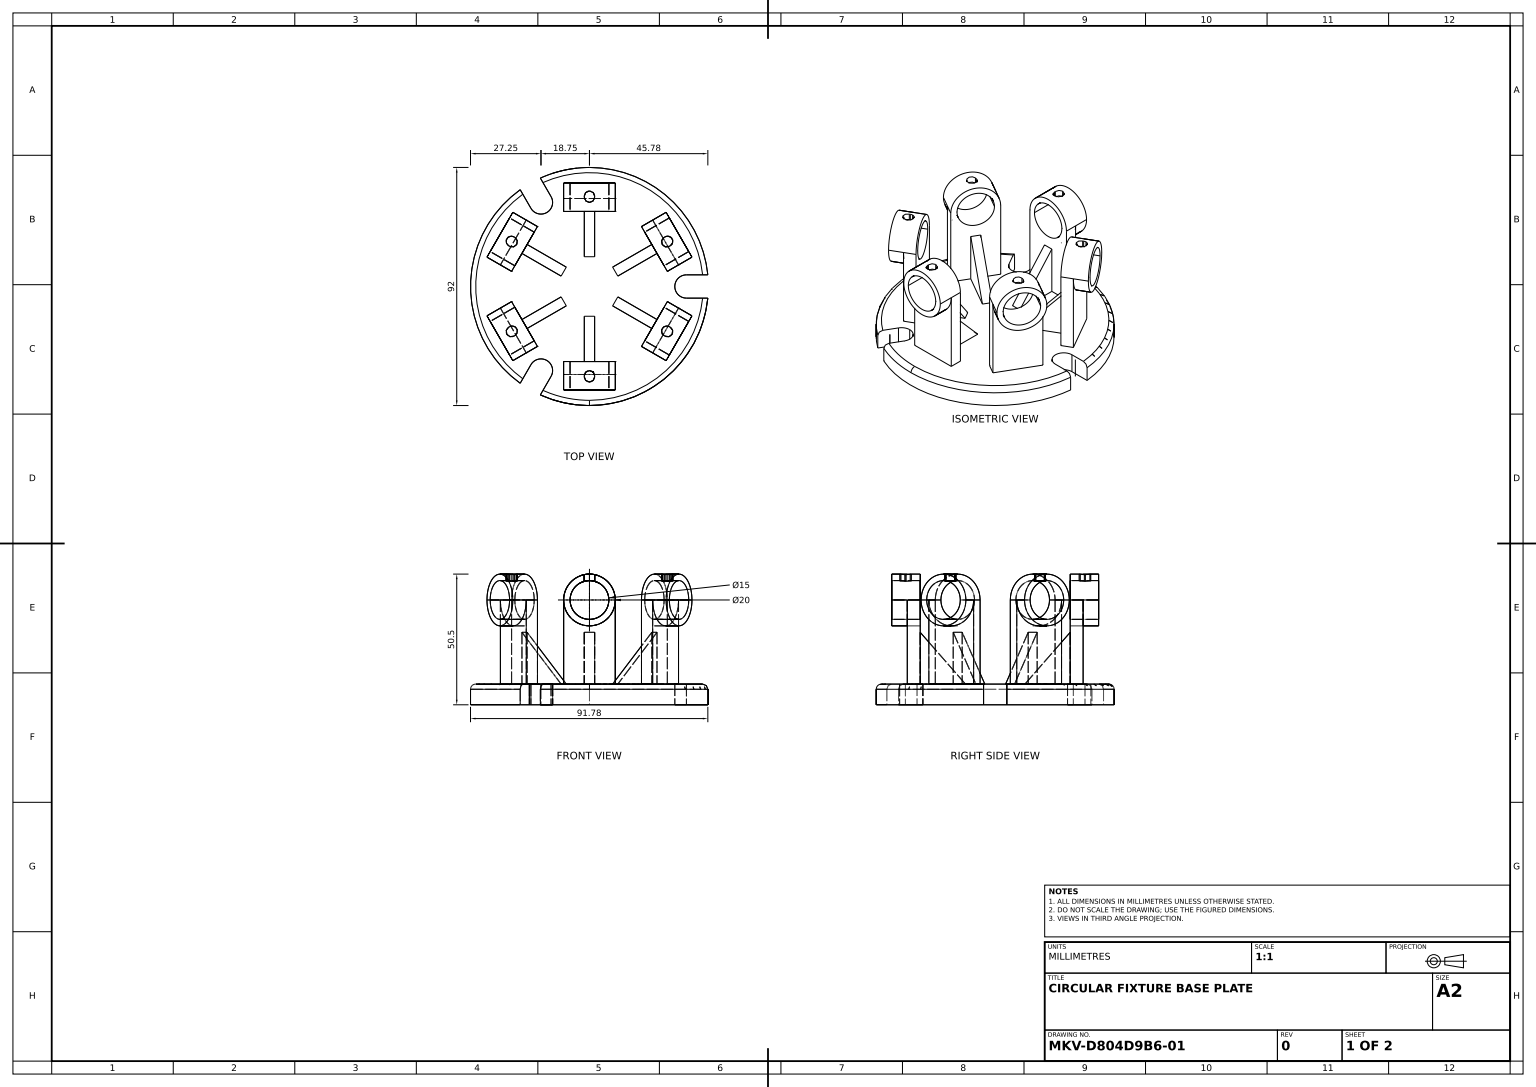
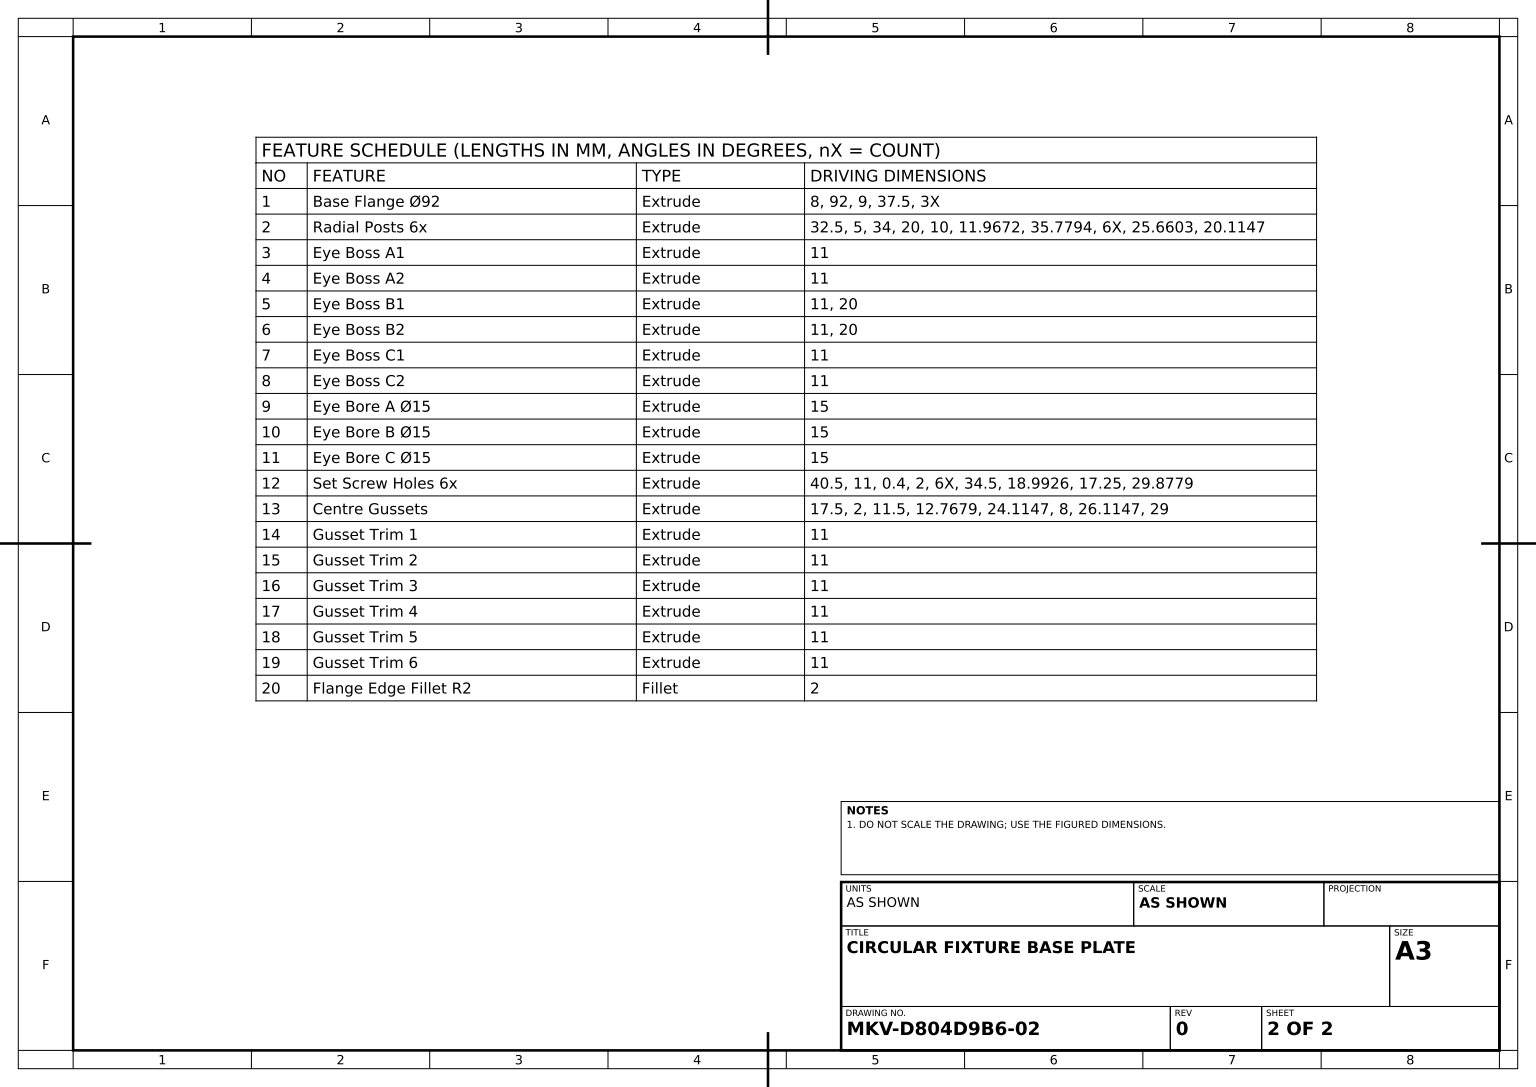
from build123d import *

# Parameters (mm, degrees)
BASE_FLANGE_92_DEPTH     = 8
RADIAL_POSTS_SKETCH_W    = 20
RADIAL_POSTS_SKETCH_H    = 5
RADIAL_POSTS_6X_DEPTH    = 32.5
EYE_BOSS_PAIR_A_SKETCH_R = 10
EYE_BOSS_A1_DEPTH        = 11
EYE_START                = 69
SKETCH6_2_R              = 10
EYE_BOSS_A2_DEPTH        = 11
EYE_BOSS_PAIR_B_SKETCH_R = 10
EYE_BOSS_B1_DEPTH        = 11
SKETCH7_2_R              = 10
EYE_BOSS_B2_DEPTH        = 11
EYE_BOSS_PAIR_C_SKETCH_R = 10
EYE_BOSS_C1_DEPTH        = 11
SKETCH8_2_R              = 10
EYE_BOSS_C2_DEPTH        = 11
EYE_BORE_A_SKETCH_R      = 7.5
EYE_BORE_A_15_DEPTH      = 110.828275048
EYE_BORE_B_SKETCH_R      = 7.5
EYE_BORE_B_15_DEPTH      = 116.644659402
EYE_BORE_C_SKETCH_R      = 7.5
EYE_BORE_C_15_DEPTH      = 116.644659402
SET_SCREW_HOLES_6X_DEPTH = 11
CENTRE_GUSSETS_SKETCH_W  = 4
CENTRE_GUSSETS_SKETCH_H  = 17.5
CENTRE_GUSSETS_DEPTH     = 20
GUSSET_TRIM_1_DEPTH      = 11
GUSSET_TRIM_2_DEPTH      = 11
GUSSET_TRIM_3_DEPTH      = 11
GUSSET_TRIM_4_DEPTH      = 11
GUSSET_TRIM_5_DEPTH      = 11
GUSSET_TRIM_6_DEPTH      = 11
FLANGE_EDGE_FILLET_R2_R  = 2


with BuildPart() as part:
    # Base Flange Sketch → Base Flange _92 (new body)
    with BuildSketch(Plane(origin=(0, 0, 0), x_dir=(1, 0, 0), z_dir=(0, 1, 0))):
        with BuildLine():
            Line((37.5, 4.5), (45.779362162, 4.5))
            ThreePointArc((45.779362162, 4.5), (23, 39.837168574), (-18.992566764, 41.896090602))
            Line((-18.992566764, 41.896090602), (-14.852885683, 34.725952642))
            ThreePointArc((-14.852885683, 34.725952642), (-16.5, 28.578838325), (-22.647114317, 30.225952642))
            Line((-22.647114317, 30.225952642), (-26.786795398, 37.396090602))
            ThreePointArc((-26.786795398, 37.396090602), (-46, 0), (-26.786795398, -37.396090602))
            Line((-26.786795398, -37.396090602), (-22.647114317, -30.225952642))
            ThreePointArc((-22.647114317, -30.225952642), (-16.5, -28.578838325), (-14.852885683, -34.725952642))
            Line((-14.852885683, -34.725952642), (-18.992566764, -41.896090602))
            ThreePointArc((-18.992566764, -41.896090602), (23, -39.837168574), (45.779362162, -4.5))
            Line((45.779362162, -4.5), (37.5, -4.5))
            ThreePointArc((37.5, -4.5), (33, 0), (37.5, 4.5))
        make_face()
    extrude(amount=BASE_FLANGE_92_DEPTH)

    # Radial Posts Sketch → Radial Posts 6x (add)
    with BuildSketch(Plane(origin=(0, 8, 0), x_dir=(1, 0, 0), z_dir=(0, 1, 0))):
        Polygon((20.11473671, 23.160254038), (30.11473671, 5.839745962), (34.444863729, 8.339745962), (24.444863729, 25.660254038), align=None)
        with Locations((0, 31.5)):
            Rectangle(RADIAL_POSTS_SKETCH_W, RADIAL_POSTS_SKETCH_H)
        Polygon((30.11473671, -5.839745962), (20.11473671, -23.160254038), (24.444863729, -25.660254038), (34.444863729, -8.339745962), align=None)
        with Locations((0, -31.5)):
            Rectangle(RADIAL_POSTS_SKETCH_W, RADIAL_POSTS_SKETCH_H)
        Polygon((-20.11473671, -23.160254038), (-30.11473671, -5.839745962), (-34.444863729, -8.339745962), (-24.444863729, -25.660254038), align=None)
        Polygon((-30.11473671, 5.839745962), (-20.11473671, 23.160254038), (-24.444863729, 25.660254038), (-34.444863729, 8.339745962), align=None)
    extrude(amount=RADIAL_POSTS_6X_DEPTH)

    # Eye Boss Pair A Sketch → Eye Boss A1 (add)
    with BuildSketch(Plane(origin=(0, 0, 29), x_dir=(-1, 0, 0), z_dir=(0, 0, -1))):
        with Locations((0, 40.5)):
            Circle(EYE_BOSS_PAIR_A_SKETCH_R)
    extrude(amount=-EYE_BOSS_A1_DEPTH)

    # Sketch6_2 → Eye Boss A2 (add)
    with BuildSketch(Plane(origin=(0, 0, 29), x_dir=(-1, 0, 0), z_dir=(0, 0, -1)).offset(EYE_START)):
        with Locations((0, 40.5)):
            Circle(SKETCH6_2_R)
    extrude(amount=-EYE_BOSS_A2_DEPTH)

    # Eye Boss Pair B Sketch → Eye Boss B1 (add)
    with BuildSketch(Plane(origin=(25.11473671, 0, -14.5), x_dir=(0.5000000000000002, 0, 0.8660254037844386), z_dir=(-0.8660254037844385, 0, 0.5000000000000001))):
        with Locations((0, 40.5)):
            Circle(EYE_BOSS_PAIR_B_SKETCH_R)
    extrude(amount=-EYE_BOSS_B1_DEPTH)

    # Sketch7_2 → Eye Boss B2 (add)
    with BuildSketch(Plane(origin=(25.11473671, 0, -14.5), x_dir=(0.5000000000000002, 0, 0.8660254037844386), z_dir=(-0.8660254037844385, 0, 0.5000000000000001)).offset(EYE_START)):
        with Locations((0, 40.5)):
            Circle(SKETCH7_2_R)
    extrude(amount=-EYE_BOSS_B2_DEPTH)

    # Eye Boss Pair C Sketch → Eye Boss C1 (add)
    with BuildSketch(Plane(origin=(25.11473671, 0, 14.5), x_dir=(-0.4999999999999997, 0, 0.8660254037844388), z_dir=(-0.8660254037844389, 0, -0.49999999999999983))):
        with Locations((0, 40.5)):
            Circle(EYE_BOSS_PAIR_C_SKETCH_R)
    extrude(amount=-EYE_BOSS_C1_DEPTH)

    # Sketch8_2 → Eye Boss C2 (add)
    with BuildSketch(Plane(origin=(25.11473671, 0, 14.5), x_dir=(-0.4999999999999997, 0, 0.8660254037844388), z_dir=(-0.8660254037844389, 0, -0.49999999999999983)).offset(EYE_START)):
        with Locations((0, 40.5)):
            Circle(SKETCH8_2_R)
    extrude(amount=-EYE_BOSS_C2_DEPTH)

    # Eye Bore A Sketch → Eye Bore A _15 (cut, through all)
    with BuildSketch(Plane.XY.offset(40)):
        with Locations((0, 40.5)):
            Circle(EYE_BORE_A_SKETCH_R)
    extrude(amount=-EYE_BORE_A_15_DEPTH, mode=Mode.SUBTRACT)

    # Eye Bore B Sketch → Eye Bore B _15 (cut, through all)
    with BuildSketch(Plane(origin=(-34.641016151, 0, 20), x_dir=(0.5000000000000004, 0, 0.8660254037844384), z_dir=(-0.8660254037844384, 0, 0.5000000000000004))):
        with Locations((0, 40.5)):
            Circle(EYE_BORE_B_SKETCH_R)
    extrude(amount=-EYE_BORE_B_15_DEPTH, mode=Mode.SUBTRACT)

    # Eye Bore C Sketch → Eye Bore C _15 (cut, through all)
    with BuildSketch(Plane(origin=(-34.641016151, 0, -20), x_dir=(-0.4999999999999995, 0, 0.866025403784439), z_dir=(-0.866025403784439, 0, -0.4999999999999995))):
        with Locations((0, 40.5)):
            Circle(EYE_BORE_C_SKETCH_R)
    extrude(amount=-EYE_BORE_C_15_DEPTH, mode=Mode.SUBTRACT)

    # Set Screw Holes Sketch → Set Screw Holes 6x (cut)
    with BuildSketch(Plane(origin=(0, 40.5, 0), x_dir=(1, 0, 0), z_dir=(0, 1, 0))):
        with BuildLine():
            Line((-2, 34.5), (-2, 34.9))
            ThreePointArc((-2, 34.9), (0, 36.9), (2, 34.9))
            Line((2, 34.9), (2, 34.5))
            ThreePointArc((2, 34.5), (0, 32.5), (-2, 34.5))
        make_face()
        with BuildLine():
            Line((28.877876431, 18.982050808), (29.224286592, 19.182050808))
            ThreePointArc((29.224286592, 19.182050808), (31.9563374, 18.45), (31.224286592, 15.717949192))
            Line((31.224286592, 15.717949192), (30.877876431, 15.517949192))
            ThreePointArc((30.877876431, 15.517949192), (28.145825623, 16.25), (28.877876431, 18.982050808))
        make_face()
        with BuildLine():
            Line((30.877876431, -15.517949192), (31.224286592, -15.717949192))
            ThreePointArc((31.224286592, -15.717949192), (31.9563374, -18.45), (29.224286592, -19.182050808))
            Line((29.224286592, -19.182050808), (28.877876431, -18.982050808))
            ThreePointArc((28.877876431, -18.982050808), (28.145825623, -16.25), (30.877876431, -15.517949192))
        make_face()
        with BuildLine():
            Line((2, -34.5), (2, -34.9))
            ThreePointArc((2, -34.9), (0, -36.9), (-2, -34.9))
            Line((-2, -34.9), (-2, -34.5))
            ThreePointArc((-2, -34.5), (0, -32.5), (2, -34.5))
        make_face()
        with BuildLine():
            Line((-28.877876431, -18.982050808), (-29.224286592, -19.182050808))
            ThreePointArc((-29.224286592, -19.182050808), (-31.9563374, -18.45), (-31.224286592, -15.717949192))
            Line((-31.224286592, -15.717949192), (-30.877876431, -15.517949192))
            ThreePointArc((-30.877876431, -15.517949192), (-28.145825623, -16.25), (-28.877876431, -18.982050808))
        make_face()
        with BuildLine():
            Line((-30.877876431, 15.517949192), (-31.224286592, 15.717949192))
            ThreePointArc((-31.224286592, 15.717949192), (-31.9563374, 18.45), (-29.224286592, 19.182050808))
            Line((-29.224286592, 19.182050808), (-28.877876431, 18.982050808))
            ThreePointArc((-28.877876431, 18.982050808), (-28.145825623, 16.25), (-30.877876431, 15.517949192))
        make_face()
    extrude(amount=SET_SCREW_HOLES_6X_DEPTH, mode=Mode.SUBTRACT)

    # Centre Gussets Sketch → Centre Gussets (add)
    with BuildSketch(Plane(origin=(0, 8, 0), x_dir=(1, 0, 0), z_dir=(0, 1, 0))):
        Polygon((-24.11473671, 16.232050808), (-26.11473671, 12.767949192), (-10.959292144, 4.017949192), (-8.959292144, 7.482050808), align=None)
        with Locations((0, 20.25)):
            Rectangle(CENTRE_GUSSETS_SKETCH_W, CENTRE_GUSSETS_SKETCH_H)
        Polygon((26.11473671, 12.767949192), (24.11473671, 16.232050808), (8.959292144, 7.482050808), (10.959292144, 4.017949192), align=None)
        Polygon((24.11473671, -16.232050808), (26.11473671, -12.767949192), (10.959292144, -4.017949192), (8.959292144, -7.482050808), align=None)
        with Locations((0, -20.25)):
            Rectangle(CENTRE_GUSSETS_SKETCH_W, CENTRE_GUSSETS_SKETCH_H)
        Polygon((-26.11473671, -12.767949192), (-24.11473671, -16.232050807), (-8.959292143, -7.482050807), (-10.959292143, -4.017949192), align=None)
    extrude(amount=CENTRE_GUSSETS_DEPTH)

    # Gusset Trim 1 Sketch → Gusset Trim 1 (cut)
    with BuildSketch(Plane(origin=(2, 0, 0), x_dir=(0, 0, -1), z_dir=(1, 0, 0))):
        Polygon((-29, 28), (-11.5, 8), (-11.5, 28), align=None)
    extrude(amount=-GUSSET_TRIM_1_DEPTH, mode=Mode.SUBTRACT)

    # Gusset Trim 2 Sketch → Gusset Trim 2 (cut)
    with BuildSketch(Plane(origin=(1, 0, 1.732050808), x_dir=(0.8660254037844386, 0, -0.5), z_dir=(0.5000000000000001, 0, 0.8660254037844387))):
        Polygon((-29, 28), (-11.5, 8), (-11.5, 28), align=None)
    extrude(amount=-GUSSET_TRIM_2_DEPTH, mode=Mode.SUBTRACT)

    # Gusset Trim 3 Sketch → Gusset Trim 3 (cut)
    with BuildSketch(Plane(origin=(-1, 0, 1.732050808), x_dir=(0.8660254037844386, 0, 0.5000000000000001), z_dir=(-0.5000000000000001, 0, 0.8660254037844386))):
        Polygon((-29, 28), (-11.5, 8), (-11.5, 28), align=None)
    extrude(amount=-GUSSET_TRIM_3_DEPTH, mode=Mode.SUBTRACT)

    # Gusset Trim 4 Sketch → Gusset Trim 4 (cut)
    with BuildSketch(Plane.ZY.offset(2)):
        Polygon((-29, 28), (-11.5, 8), (-11.5, 28), align=None)
    extrude(amount=-GUSSET_TRIM_4_DEPTH, mode=Mode.SUBTRACT)

    # Gusset Trim 5 Sketch → Gusset Trim 5 (cut)
    with BuildSketch(Plane(origin=(-1, 0, -1.732050808), x_dir=(-0.8660254037844386, 0, 0.5000000000000001), z_dir=(-0.5000000000000001, 0, -0.8660254037844386))):
        Polygon((-29, 28), (-11.5, 8), (-11.5, 28), align=None)
    extrude(amount=-GUSSET_TRIM_5_DEPTH, mode=Mode.SUBTRACT)

    # Gusset Trim 6 Sketch → Gusset Trim 6 (cut)
    with BuildSketch(Plane(origin=(1, 0, -1.732050808), x_dir=(-0.8660254037844388, 0, -0.4999999999999997), z_dir=(0.4999999999999997, 0, -0.8660254037844388))):
        Polygon((-29, 28), (-11.5, 8), (-11.5, 28), align=None)
    extrude(amount=-GUSSET_TRIM_6_DEPTH, mode=Mode.SUBTRACT)

    # Flange Edge Fillet R2
    flange_edge_fillet_r2_edges = [part.edges().sort_by_distance(p)[0] for p in [
        (23, 8, -39.837168574),
        (-46, 8, 0),
        (23, 8, 39.837168574),
    ]]
    fillet(flange_edge_fillet_r2_edges, radius=FLANGE_EDGE_FILLET_R2_R)


solid = part.part
